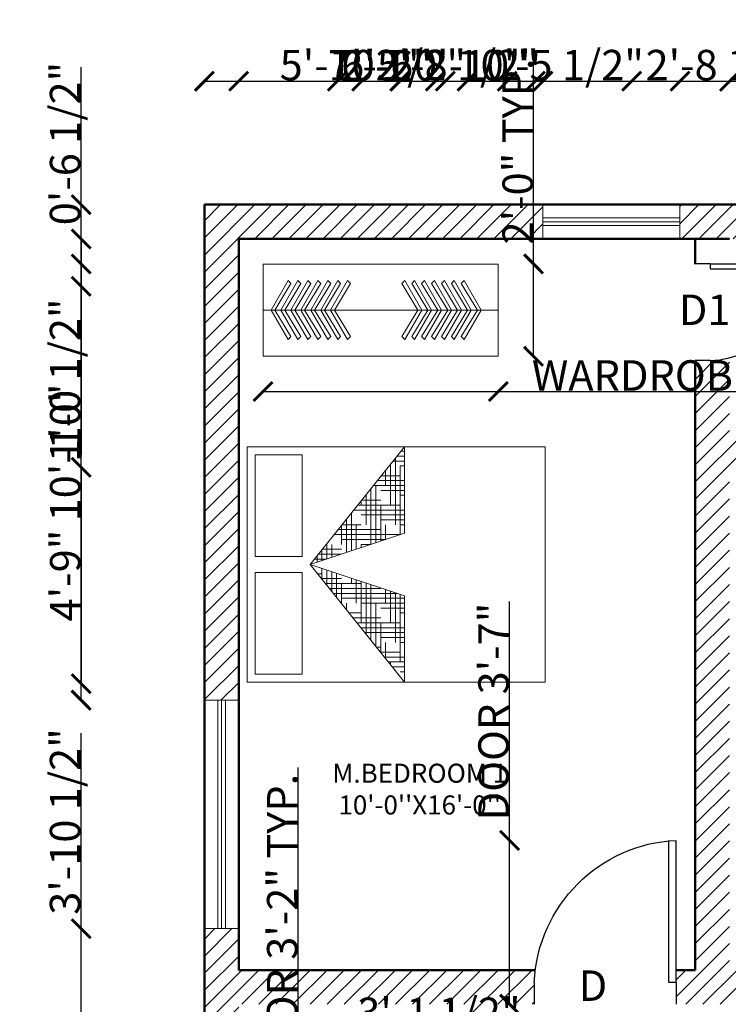
# Model space of a CAD drawing. Units: inches. Extents: x 1385 to 1778, y 1343 to 2100.
# Tile 4 of 6: x 1385 to 1571, y 1821 to 2079. Entities that reach past the tile are written whole.
import ezdxf

# ---------------------------------------------------------------- set-up
doc = ezdxf.new("R2010")
doc.units = ezdxf.units.IN
for name, color, linetype, lineweight in [('A-ANNO-DIMS', 2, 'Continuous', 18), ('A-ANNO-TEXT', 7, 'Continuous', 25), ('A-AREA-IDEN', 7, 'Continuous', 25), ('A-FURN', 8, 'Continuous', 18), ('A-WALL-PATT', 8, 'Continuous', 13), ('Door', 150, 'Continuous', 25), ('Wall', 7, 'Continuous', 50), ('Wardrobe', 114, 'Continuous', 18), ('Windows', 140, 'Continuous', 18)]:
    doc.layers.add(name, color=color, linetype=linetype, lineweight=lineweight)
doc.styles.get("Standard").update_dxf_attribs({"font": 'arial.ttf'})
doc.dimstyles.get("Standard").update_dxf_attribs({"dimtxt": 8, "dimasz": 5, "dimexe": 0.18, "dimexo": 0.0625, "dimgap": 0.09, "dimtad": 1, "dimdec": 1, "dimzin": 0, "dimdsep": 46, "dimlunit": 4, "dimtxsty": 'Standard', "dimblk": 'ARCHTICK', "dimcen": 0.09, "dimse1": 1, "dimse2": 1, "dimadec": 0, "dimazin": 0, "dimtfac": 1, "dimtdec": 1, "dimtofl": 0, "dimtmove": 0, "dimatfit": 3, "dimfxl": 1, "dimtolj": 1, "dimtzin": 0, "dimarcsym": 0})

# ---------------------------------------------------------------- blocks, each defined once
blk = doc.blocks.new('AP0B05')
for p, q in [((35, 100), (35, 880)), ((75, 100), (75, 878.9)), ((35, 100), (35, -20)), ((815, 100), (815, -20))]:
    blk.add_line(p, q)
blk.add_lwpolyline([(35, 100), (75, 100)])
blk.add_arc((-2.4, 62.6), 818.3, 2.6212, 87.3788)
blk = doc.blocks.new('*X10')
at = {"color": 0}
for p, q in [((20.25, 14.8125), (20.2772, 14.8125)), ((20.1739, 14.75), (20.2772, 14.75)), ((20.1875, 14.75), (20.1875, 14.7669)), ((20.199, 14.7812), (20.2772, 14.7812)), ((20.25, 14.3194), (20.25, 14.75)), ((20.1236, 14.6875), (20.25, 14.6875)), ((20.125, 14.5), (20.125, 14.6893)), ((20.1487, 14.7188), (20.2772, 14.7188)), ((20.1562, 14.625), (20.1562, 14.7281)), ((20.0938, 14.375), (20.0938, 14.6504)), ((20.0984, 14.6562), (20.125, 14.6562)), ((20.2188, 14.3091), (20.2188, 14.625)), ((20.25, 14.625), (20.2772, 14.625)), ((20.023, 14.5625), (20.2772, 14.5625)), ((20.0312, 14.2469), (20.0312, 14.5727)), ((20.0625, 14.2573), (20.0625, 14.6116)), ((20.125, 14.5938), (20.2772, 14.5938)), ((19.9727, 14.5), (20.25, 14.5)), ((19.9979, 14.5312), (20.2772, 14.5312)), ((20, 14.2366), (20, 14.5)), ((20.1875, 14.2987), (20.1875, 14.5)), ((19.9225, 14.4375), (20, 14.4375)), ((19.9476, 14.4688), (20.125, 14.4688)), ((20.25, 14.4375), (20.2772, 14.4375)), ((19.875, 14.25), (19.875, 14.3785)), ((19.9062, 14.375), (19.9062, 14.4174)), ((19.9688, 14.2262), (19.9688, 14.375)), ((20, 14.375), (20.2772, 14.375)), ((20.125, 14.4062), (20.2772, 14.4062)), ((20.1562, 14.2884), (20.1562, 14.375)), ((19.8219, 14.3125), (20.2291, 14.3125)), ((19.8438, 14.1848), (19.8438, 14.3397)), ((19.875, 14.3438), (20.2772, 14.3438)), ((19.7716, 14.25), (20, 14.25)), ((19.7812, 14.1641), (19.7812, 14.262)), ((19.7967, 14.2812), (20.125, 14.2812)), ((19.8125, 14.1744), (19.8125, 14.3008)), ((19.9375, 14.2159), (19.9375, 14.25)), ((19.7213, 14.1875), (19.75, 14.1875)), ((19.7465, 14.2188), (19.875, 14.2188)), ((19.75, 14.1537), (19.75, 14.2231)), ((19.7018, 14.0938), (19.7786, 14.0938)), ((19.7188, 14.0726), (19.7188, 14.1136)), ((19.7269, 14.0625), (19.8728, 14.0625)), ((19.75, 14.0338), (19.75, 14.1032)), ((19.7812, 13.9949), (19.7812, 14.0929)), ((19.8125, 14), (19.8125, 14.0825)), ((19.752, 14.0312), (19.875, 14.0312)), ((19.875, 13.8784), (19.875, 14)), ((19.9062, 13.8396), (19.9062, 14.0514)), ((19.9375, 13.8007), (19.9375, 14.0411)), ((19.9688, 13.875), (19.9688, 14.0307)), ((20, 14), (20, 14.0204)), ((20, 14), (20.0614, 14)), ((20.0625, 13.6454), (20.0625, 13.9996)), ((19.8275, 13.9375), (20.25, 13.9375)), ((19.875, 13.9688), (20.1557, 13.9688)), ((20.0938, 13.625), (20.0938, 13.9893)), ((20.125, 13.75), (20.125, 13.9789)), ((20.1562, 13.875), (20.1562, 13.9686)), ((20.25, 13.5), (20.25, 13.9375)), ((19.8526, 13.9062), (20.125, 13.9062)), ((19.8777, 13.875), (20, 13.875)), ((20.0312, 13.6842), (20.0312, 13.875)), ((20.2188, 13.4511), (20.2188, 13.875)), ((20.25, 13.875), (20.2772, 13.875)), ((20, 13.8125), (20.2772, 13.8125)), ((20.125, 13.8438), (20.2772, 13.8438)), ((19.9532, 13.7812), (20.2772, 13.7812)), ((19.9783, 13.75), (20.25, 13.75)), ((20, 13.723), (20, 13.75)), ((20.1875, 13.49), (20.1875, 13.75)), ((20.0035, 13.7188), (20.125, 13.7188)), ((20.25, 13.6875), (20.2772, 13.6875)), ((20.0789, 13.625), (20.2772, 13.625)), ((20.125, 13.6562), (20.2772, 13.6562)), ((20.1562, 13.5288), (20.1562, 13.625)), ((20.104, 13.5938), (20.2772, 13.5938)), ((20.1292, 13.5625), (20.25, 13.5625)), ((20.25, 13.5), (20.2772, 13.5)), ((20.2046, 13.4688), (20.2772, 13.4688)), ((20.2297, 13.4375), (20.2772, 13.4375)), ((20.2549, 13.4062), (20.2772, 13.4062))]:
    blk.add_line(p, q, dxfattribs=at)
blk = doc.blocks.new('MAT-P13')
for p, q in [((-0.75, 0), (0.75, 0)), ((-0.75, 0), (-0.75, -1.9)), ((0.75, 0), (0.75, -1.9)), ((-0.7, -0.05), (-0.7, -0.35)), ((-0.7, -0.05), (-0.05, -0.05)), ((-0.05, -0.35), (-0.05, -0.05)), ((0.05, -0.05), (0.7, -0.05)), ((0.05, -0.35), (0.05, -0.05)), ((0.7, -0.05), (0.7, -0.35)), ((-0.7, -0.35), (-0.05, -0.35)), ((0.05, -0.35), (0.7, -0.35)), ((-0.75, -1.0034), (0, -0.4)), ((0, -0.4), (-0.75, -1.0034)), ((0, -0.4), (-0.2, -1.0034)), ((0, -0.4), (0.2, -1.0034)), ((0, -0.4), (0.75, -1.0034)), ((-0.75, -1.0034), (-0.2, -1.0034)), ((0.2, -1.0034), (0.75, -1.0034)), ((0.75, -1.9), (-0.75, -1.9))]:
    blk.add_line(p, q)
at = {"xscale": -1, "rotation": 90}
blk.add_blockref('*X10', (14.1285, 19.2738), dxfattribs=at)
blk = doc.blocks.new('WARDROBE-DOUBLE')
blk.add_line((0, 12.12), (61.84, 12.12))
blk.add_lwpolyline([(0, 24.24), (61.84, 24.24), (61.84, 0), (0, 0)], close=True)
for points in [[(2.11, 12.12), (6.58, 19.87), (7.34, 19.08), (3.11, 12.12)], [(4.72, 12.12), (9.19, 19.87), (9.95, 19.08), (5.72, 12.12)], [(7.33, 12.12), (11.8, 19.87), (12.56, 19.08), (8.32, 12.12)], [(9.94, 12.12), (14.41, 19.87), (15.17, 19.08), (10.93, 12.12)], [(12.54, 12.12), (17.02, 19.87), (17.78, 19.08), (13.54, 12.12)], [(15.15, 12.12), (19.62, 19.87), (20.38, 19.08), (16.15, 12.12)], [(17.76, 12.12), (22.23, 19.87), (22.99, 19.08), (18.76, 12.12)], [(41.7, 12.12), (37.23, 19.87), (36.47, 19.08), (40.7, 12.12)], [(44.31, 12.12), (39.83, 19.87), (39.07, 19.08), (43.31, 12.12)], [(46.91, 12.12), (42.44, 19.87), (41.68, 19.08), (45.92, 12.12)], [(49.52, 12.12), (45.05, 19.87), (44.29, 19.08), (48.53, 12.12)], [(52.13, 12.12), (47.66, 19.87), (46.9, 19.08), (51.13, 12.12)], [(54.74, 12.12), (50.27, 19.87), (49.51, 19.08), (53.74, 12.12)], [(57.35, 12.12), (52.88, 19.87), (52.12, 19.08), (56.35, 12.12)], [(2.11, 12.12), (6.58, 4.38), (7.34, 5.17), (3.11, 12.12)], [(4.72, 12.12), (9.19, 4.38), (9.95, 5.17), (5.72, 12.12)], [(7.33, 12.12), (11.8, 4.38), (12.56, 5.17), (8.32, 12.12)], [(9.94, 12.12), (14.41, 4.38), (15.17, 5.17), (10.93, 12.12)], [(12.54, 12.12), (17.02, 4.38), (17.78, 5.17), (13.54, 12.12)], [(15.15, 12.12), (19.62, 4.38), (20.38, 5.17), (16.15, 12.12)], [(17.76, 12.12), (22.23, 4.38), (22.99, 5.17), (18.76, 12.12)], [(41.7, 12.12), (37.23, 4.38), (36.47, 5.17), (40.7, 12.12)], [(44.31, 12.12), (39.83, 4.38), (39.07, 5.17), (43.31, 12.12)], [(46.91, 12.12), (42.44, 4.38), (41.68, 5.17), (45.92, 12.12)], [(49.52, 12.12), (45.05, 4.38), (44.29, 5.17), (48.53, 12.12)], [(52.13, 12.12), (47.66, 4.38), (46.9, 5.17), (51.13, 12.12)], [(54.74, 12.12), (50.27, 4.38), (49.51, 5.17), (53.74, 12.12)], [(57.35, 12.12), (52.88, 4.38), (52.12, 5.17), (56.35, 12.12)]]:
    blk.add_lwpolyline(points)
blk = doc.blocks.new('WINDOW-GLAZING-36IN')
for p, q in [((0, 0), (0, 36)), ((1, 0), (1, 36)), ((2, 0), (2, 36))]:
    blk.add_line(p, q)
blk = doc.blocks.new('WINDOW-GLAZING-60IN')
for p, q in [((0, 0), (0, 60)), ((1, 0), (1, 60)), ((2, 0), (2, 60))]:
    blk.add_line(p, q)
blk = doc.blocks.new('_ArchTick')
at = {"color": 0, "linetype": 'ByBlock', "const_width": 0.15}
blk.add_lwpolyline([(-0.5, -0.5), (0.5, 0.5)], dxfattribs=at)
blk = doc.blocks.new('*D19')
at = {"layer": 'A-ANNO-DIMS', "color": 0, "lineweight": -2, "transparency": 16777216}
for p, q in [((1458.44, 1792.72), (1458.44, 1882.9)), ((1458.44, 1754.73), (1458.44, 1792.72))]:
    blk.add_line(p, q, dxfattribs=at)
at = {"layer": 'Defpoints', "color": 0, "transparency": 16777216}
for p in [(1458.44, 1792.72), (1464.14, 1792.72), (1464.14, 1754.73)]:
    blk.add_point(p, dxfattribs=at)
at = {"layer": 'A-ANNO-DIMS', "color": 0, "lineweight": -2, "transparency": 16777216, "xscale": 5, "yscale": 5, "zscale": 5}
for p, rotation in [((1458.44, 1792.72), 90), ((1458.44, 1754.73), 270)]:
    blk.add_blockref('_ArchTick', p, dxfattribs=dict(at, rotation=rotation))
at = {"layer": 'A-ANNO-DIMS', "color": 0, "transparency": 16777216, "insert": (1454.21, 1840.31), "char_height": 8, "attachment_point": 5, "rotation": 90}
blk.add_mtext('\\A1;DOOR 3\'-2" TYP.', dxfattribs=at)
blk = doc.blocks.new('*D21')
at = {"layer": 'A-ANNO-DIMS', "color": 0, "lineweight": -2, "transparency": 16777216}
for p, q in [((1513.99, 1863.79), (1513.99, 1926.47)), ((1513.99, 1820.73), (1513.99, 1863.79))]:
    blk.add_line(p, q, dxfattribs=at)
at = {"layer": 'Defpoints', "color": 0, "transparency": 16777216}
for p in [(1513.99, 1863.79), (1520.45, 1863.79), (1520.45, 1820.73)]:
    blk.add_point(p, dxfattribs=at)
at = {"layer": 'A-ANNO-DIMS', "color": 0, "lineweight": -2, "transparency": 16777216, "xscale": 5, "yscale": 5, "zscale": 5}
for p, rotation in [((1513.99, 1863.79), 90), ((1513.99, 1820.73), 270)]:
    blk.add_blockref('_ArchTick', p, dxfattribs=dict(at, rotation=rotation))
at = {"layer": 'A-ANNO-DIMS', "color": 0, "transparency": 16777216, "insert": (1509.76, 1897.63), "char_height": 8, "attachment_point": 5, "rotation": 90}
blk.add_mtext('\\A1;DOOR 3\'-7"', dxfattribs=at)
blk = doc.blocks.new('*D22')
at = {"layer": 'A-ANNO-DIMS', "color": 0, "lineweight": -2, "transparency": 16777216}
for p, q in [((1520.45, 1814.28), (1475.37, 1814.28)), ((1557.76, 1814.28), (1520.45, 1814.28))]:
    blk.add_line(p, q, dxfattribs=at)
at = {"layer": 'Defpoints', "color": 0, "transparency": 16777216}
for p in [(1520.45, 1820.73), (1557.76, 1820.73), (1520.45, 1814.28)]:
    blk.add_point(p, dxfattribs=at)
at = {"layer": 'A-ANNO-DIMS', "color": 0, "lineweight": -2, "transparency": 16777216, "xscale": 5, "yscale": 5, "zscale": 5, "rotation": 180}
blk.add_blockref('_ArchTick', (1520.45, 1814.28), dxfattribs=at)
at = {"layer": 'A-ANNO-DIMS', "color": 0, "lineweight": -2, "transparency": 16777216, "xscale": 5, "yscale": 5, "zscale": 5}
blk.add_blockref('_ArchTick', (1557.76, 1814.28), dxfattribs=at)
at = {"layer": 'A-ANNO-DIMS', "color": 0, "transparency": 16777216, "insert": (1495.41, 1818.51), "char_height": 8, "attachment_point": 5}
blk.add_mtext('\\A1;3\'-1 1/2"', dxfattribs=at)
blk = doc.blocks.new('*D37')
at = {"layer": 'A-ANNO-DIMS', "color": 0, "lineweight": -2, "transparency": 16777216}
for p, q in [((1449.17, 1981.63), (1511.01, 1981.63)), ((1511.01, 1981.63), (1634.21, 1981.63))]:
    blk.add_line(p, q, dxfattribs=at)
at = {"layer": 'Defpoints', "color": 0, "transparency": 16777216}
for p in [(1449.17, 1990.9), (1511.01, 1990.9), (1511.01, 1981.63)]:
    blk.add_point(p, dxfattribs=at)
at = {"layer": 'A-ANNO-DIMS', "color": 0, "lineweight": -2, "transparency": 16777216, "xscale": 5, "yscale": 5, "zscale": 5, "rotation": 180}
blk.add_blockref('_ArchTick', (1449.17, 1981.63), dxfattribs=at)
at = {"layer": 'A-ANNO-DIMS', "color": 0, "lineweight": -2, "transparency": 16777216, "xscale": 5, "yscale": 5, "zscale": 5}
blk.add_blockref('_ArchTick', (1511.01, 1981.63), dxfattribs=at)
at = {"layer": 'A-ANNO-DIMS', "color": 0, "transparency": 16777216, "insert": (1575.11, 1985.86), "char_height": 8, "attachment_point": 5}
blk.add_mtext('\\A1;WARDROBE 5\'-2" TYP.', dxfattribs=at)
blk = doc.blocks.new('*D38')
at = {"layer": 'A-ANNO-DIMS', "color": 0, "lineweight": -2, "transparency": 16777216}
for p, q in [((1520.29, 2015.15), (1520.29, 2069.23)), ((1520.29, 1990.9), (1520.29, 2015.15))]:
    blk.add_line(p, q, dxfattribs=at)
at = {"layer": 'Defpoints', "color": 0, "transparency": 16777216}
for p in [(1511.01, 2015.15), (1520.29, 2015.15), (1511.01, 1990.9)]:
    blk.add_point(p, dxfattribs=at)
at = {"layer": 'A-ANNO-DIMS', "color": 0, "lineweight": -2, "transparency": 16777216, "xscale": 5, "yscale": 5, "zscale": 5}
for p, rotation in [((1520.29, 2015.15), 90), ((1520.29, 1990.9), 270)]:
    blk.add_blockref('_ArchTick', p, dxfattribs=dict(at, rotation=rotation))
at = {"layer": 'A-ANNO-DIMS', "color": 0, "transparency": 16777216, "insert": (1516.11, 2044.69), "char_height": 8, "attachment_point": 5, "rotation": 90}
blk.add_mtext('\\A1;2\'-0" TYP.', dxfattribs=at)
blk = doc.blocks.new('*D51')
at = {"layer": 'A-ANNO-DIMS', "color": 0, "lineweight": -2, "transparency": 16777216}
blk.add_line((1433.77, 2063.14), (1522.75, 2063.14), dxfattribs=at)
at = {"layer": 'Defpoints', "color": 0, "transparency": 16777216}
for p in [(1522.75, 2063.14), (1433.77, 2030.73), (1522.75, 2030.73)]:
    blk.add_point(p, dxfattribs=at)
at = {"layer": 'A-ANNO-DIMS', "color": 0, "lineweight": -2, "transparency": 16777216, "xscale": 5, "yscale": 5, "zscale": 5, "rotation": 180}
blk.add_blockref('_ArchTick', (1433.77, 2063.14), dxfattribs=at)
at = {"layer": 'A-ANNO-DIMS', "color": 0, "lineweight": -2, "transparency": 16777216, "xscale": 5, "yscale": 5, "zscale": 5}
blk.add_blockref('_ArchTick', (1522.75, 2063.14), dxfattribs=at)
at = {"layer": 'A-ANNO-DIMS', "color": 0, "transparency": 16777216, "insert": (1478.26, 2067.3), "char_height": 8, "attachment_point": 5}
blk.add_mtext('\\A1;7\'-5"', dxfattribs=at)
blk = doc.blocks.new('*D52')
at = {"layer": 'A-ANNO-DIMS', "color": 0, "lineweight": -2, "transparency": 16777216}
for p, q in [((1558.75, 2063.14), (1591.32, 2063.14)), ((1591.32, 2063.14), (1636.55, 2063.14))]:
    blk.add_line(p, q, dxfattribs=at)
at = {"layer": 'Defpoints', "color": 0, "transparency": 16777216}
for p in [(1591.32, 2063.14), (1558.75, 2030.73), (1591.32, 2030.73)]:
    blk.add_point(p, dxfattribs=at)
at = {"layer": 'A-ANNO-DIMS', "color": 0, "lineweight": -2, "transparency": 16777216, "xscale": 5, "yscale": 5, "zscale": 5, "rotation": 180}
blk.add_blockref('_ArchTick', (1558.75, 2063.14), dxfattribs=at)
at = {"layer": 'A-ANNO-DIMS', "color": 0, "lineweight": -2, "transparency": 16777216, "xscale": 5, "yscale": 5, "zscale": 5}
blk.add_blockref('_ArchTick', (1591.32, 2063.14), dxfattribs=at)
at = {"layer": 'A-ANNO-DIMS', "color": 0, "transparency": 16777216, "insert": (1616.44, 2067.37), "char_height": 8, "attachment_point": 5}
blk.add_mtext('\\A1;2\'-8 1/2"', dxfattribs=at)
blk = doc.blocks.new('*D54')
at = {"layer": 'A-ANNO-DIMS', "color": 0, "lineweight": -2, "transparency": 16777216}
blk.add_line((1401.37, 1961.73), (1401.37, 1904.94), dxfattribs=at)
at = {"layer": 'Defpoints', "color": 0, "transparency": 16777216}
for p in [(1718.77, 1961.73), (1401.37, 1904.94), (1718.77, 1904.94)]:
    blk.add_point(p, dxfattribs=at)
at = {"layer": 'A-ANNO-DIMS', "color": 0, "lineweight": -2, "transparency": 16777216, "xscale": 5, "yscale": 5, "zscale": 5}
for p, rotation in [((1401.37, 1961.73), 90), ((1401.37, 1904.94), 270)]:
    blk.add_blockref('_ArchTick', p, dxfattribs=dict(at, rotation=rotation))
at = {"layer": 'A-ANNO-DIMS', "color": 0, "transparency": 16777216, "insert": (1397.19, 1933.34), "char_height": 8, "attachment_point": 5, "rotation": 90}
blk.add_mtext('\\A1;4\'-9"', dxfattribs=at)
blk = doc.blocks.new('*D56')
at = {"layer": 'A-ANNO-DIMS', "color": 0, "lineweight": -2, "transparency": 16777216}
blk.add_line((1401.37, 1900.6), (1401.37, 2030.73), dxfattribs=at)
at = {"layer": 'Defpoints', "color": 0, "transparency": 16777216}
for p in [(1401.37, 2030.73), (1433.77, 2030.73), (1433.77, 1900.6)]:
    blk.add_point(p, dxfattribs=at)
at = {"layer": 'A-ANNO-DIMS', "color": 0, "lineweight": -2, "transparency": 16777216, "xscale": 5, "yscale": 5, "zscale": 5}
for p, rotation in [((1401.37, 2030.73), 90), ((1401.37, 1900.6), 270)]:
    blk.add_blockref('_ArchTick', p, dxfattribs=dict(at, rotation=rotation))
at = {"layer": 'A-ANNO-DIMS', "color": 0, "transparency": 16777216, "insert": (1397.19, 1965.67), "char_height": 8, "attachment_point": 5, "rotation": 90}
blk.add_mtext('\\A1;10\'-10"', dxfattribs=at)
blk = doc.blocks.new('*D57')
at = {"layer": 'A-ANNO-DIMS', "color": 0, "lineweight": -2, "transparency": 16777216}
for p, q in [((1401.37, 1840.6), (1401.37, 1891.9)), ((1401.37, 1794.33), (1401.37, 1840.6))]:
    blk.add_line(p, q, dxfattribs=at)
at = {"layer": 'Defpoints', "color": 0, "transparency": 16777216}
for p in [(1401.37, 1840.6), (1433.77, 1840.6), (1433.77, 1794.33)]:
    blk.add_point(p, dxfattribs=at)
at = {"layer": 'A-ANNO-DIMS', "color": 0, "lineweight": -2, "transparency": 16777216, "xscale": 5, "yscale": 5, "zscale": 5}
for p, rotation in [((1401.37, 1840.6), 90), ((1401.37, 1794.33), 270)]:
    blk.add_blockref('_ArchTick', p, dxfattribs=dict(at, rotation=rotation))
at = {"layer": 'A-ANNO-DIMS', "color": 0, "transparency": 16777216, "insert": (1397.14, 1868.75), "char_height": 8, "attachment_point": 5, "rotation": 90}
blk.add_mtext('\\A1;3\'-10 1/2"', dxfattribs=at)
blk = doc.blocks.new('*D62')
at = {"layer": 'A-ANNO-DIMS', "color": 0, "lineweight": -2, "transparency": 16777216}
for p, q in [((1442.77, 2063.14), (1475.11, 2063.14)), ((1475.11, 2063.14), (1520.34, 2063.14))]:
    blk.add_line(p, q, dxfattribs=at)
at = {"layer": 'Defpoints', "color": 0, "transparency": 16777216}
for p in [(1475.11, 2063.14), (1442.77, 1391.73), (1475.11, 1391.73)]:
    blk.add_point(p, dxfattribs=at)
at = {"layer": 'A-ANNO-DIMS', "color": 0, "lineweight": -2, "transparency": 16777216, "xscale": 5, "yscale": 5, "zscale": 5, "rotation": 180}
blk.add_blockref('_ArchTick', (1442.77, 2063.14), dxfattribs=at)
at = {"layer": 'A-ANNO-DIMS', "color": 0, "lineweight": -2, "transparency": 16777216, "xscale": 5, "yscale": 5, "zscale": 5}
blk.add_blockref('_ArchTick', (1475.11, 2063.14), dxfattribs=at)
at = {"layer": 'A-ANNO-DIMS', "color": 0, "transparency": 16777216, "insert": (1500.22, 2067.37), "char_height": 8, "attachment_point": 5}
blk.add_mtext('\\A1;2\'-8 1/2"', dxfattribs=at)
blk = doc.blocks.new('*D63')
at = {"layer": 'A-ANNO-DIMS', "color": 0, "lineweight": -2, "transparency": 16777216}
for p, q in [((1475.11, 2063.14), (1485.11, 2063.14)), ((1485.11, 2063.14), (1517.77, 2063.14))]:
    blk.add_line(p, q, dxfattribs=at)
at = {"layer": 'Defpoints', "color": 0, "transparency": 16777216}
for p in [(1485.11, 2063.14), (1475.11, 1391.73), (1485.11, 1391.73)]:
    blk.add_point(p, dxfattribs=at)
at = {"layer": 'A-ANNO-DIMS', "color": 0, "lineweight": -2, "transparency": 16777216, "xscale": 5, "yscale": 5, "zscale": 5, "rotation": 180}
blk.add_blockref('_ArchTick', (1475.11, 2063.14), dxfattribs=at)
at = {"layer": 'A-ANNO-DIMS', "color": 0, "lineweight": -2, "transparency": 16777216, "xscale": 5, "yscale": 5, "zscale": 5}
blk.add_blockref('_ArchTick', (1485.11, 2063.14), dxfattribs=at)
at = {"layer": 'A-ANNO-DIMS', "color": 0, "transparency": 16777216, "insert": (1503.94, 2067.31), "char_height": 8, "attachment_point": 5}
blk.add_mtext('\\A1;0\'-10"', dxfattribs=at)
blk = doc.blocks.new('*D66')
at = {"layer": 'A-ANNO-DIMS', "color": 0, "lineweight": -2, "transparency": 16777216}
blk.add_line((1442.77, 2063.14), (1513.34, 2063.14), dxfattribs=at)
at = {"layer": 'Defpoints', "color": 0, "transparency": 16777216}
for p in [(1513.34, 2063.14), (1442.77, 1595.73), (1513.34, 1595.73)]:
    blk.add_point(p, dxfattribs=at)
at = {"layer": 'A-ANNO-DIMS', "color": 0, "lineweight": -2, "transparency": 16777216, "xscale": 5, "yscale": 5, "zscale": 5, "rotation": 180}
blk.add_blockref('_ArchTick', (1442.77, 2063.14), dxfattribs=at)
at = {"layer": 'A-ANNO-DIMS', "color": 0, "lineweight": -2, "transparency": 16777216, "xscale": 5, "yscale": 5, "zscale": 5}
blk.add_blockref('_ArchTick', (1513.34, 2063.14), dxfattribs=at)
at = {"layer": 'A-ANNO-DIMS', "color": 0, "transparency": 16777216, "insert": (1478.05, 2067.37), "char_height": 8, "attachment_point": 5}
blk.add_mtext('\\A1;5\'-10 1/2"', dxfattribs=at)
blk = doc.blocks.new('*D67')
at = {"layer": 'A-ANNO-DIMS', "color": 0, "lineweight": -2, "transparency": 16777216}
for p, q in [((1513.34, 2063.14), (1546.08, 2063.14)), ((1546.08, 2063.14), (1591.31, 2063.14))]:
    blk.add_line(p, q, dxfattribs=at)
at = {"layer": 'Defpoints', "color": 0, "transparency": 16777216}
for p in [(1546.08, 2063.14), (1513.34, 1595.73), (1546.08, 1595.73)]:
    blk.add_point(p, dxfattribs=at)
at = {"layer": 'A-ANNO-DIMS', "color": 0, "lineweight": -2, "transparency": 16777216, "xscale": 5, "yscale": 5, "zscale": 5, "rotation": 180}
blk.add_blockref('_ArchTick', (1513.34, 2063.14), dxfattribs=at)
at = {"layer": 'A-ANNO-DIMS', "color": 0, "lineweight": -2, "transparency": 16777216, "xscale": 5, "yscale": 5, "zscale": 5}
blk.add_blockref('_ArchTick', (1546.08, 2063.14), dxfattribs=at)
at = {"layer": 'A-ANNO-DIMS', "color": 0, "transparency": 16777216, "insert": (1571.19, 2067.37), "char_height": 8, "attachment_point": 5}
blk.add_mtext('\\A1;2\'-8 1/2"', dxfattribs=at)
blk = doc.blocks.new('*D69')
at = {"layer": 'A-ANNO-DIMS', "color": 0, "lineweight": -2, "transparency": 16777216}
blk.add_line((1442.77, 2063.14), (1520.74, 2063.14), dxfattribs=at)
at = {"layer": 'Defpoints', "color": 0, "transparency": 16777216}
for p in [(1520.74, 2063.14), (1442.77, 1829.73), (1520.74, 1829.73)]:
    blk.add_point(p, dxfattribs=at)
at = {"layer": 'A-ANNO-DIMS', "color": 0, "lineweight": -2, "transparency": 16777216, "xscale": 5, "yscale": 5, "zscale": 5, "rotation": 180}
blk.add_blockref('_ArchTick', (1442.77, 2063.14), dxfattribs=at)
at = {"layer": 'A-ANNO-DIMS', "color": 0, "lineweight": -2, "transparency": 16777216, "xscale": 5, "yscale": 5, "zscale": 5}
blk.add_blockref('_ArchTick', (1520.74, 2063.14), dxfattribs=at)
at = {"layer": 'A-ANNO-DIMS', "color": 0, "transparency": 16777216, "insert": (1481.75, 2067.31), "char_height": 8, "attachment_point": 5}
blk.add_mtext('\\A1;6\'-6"', dxfattribs=at)
blk = doc.blocks.new('*D70')
at = {"layer": 'A-ANNO-DIMS', "color": 0, "lineweight": -2, "transparency": 16777216}
for p, q in [((1571.77, 2063.14), (1578.09, 2063.14)), ((1578.09, 2063.14), (1623.18, 2063.14))]:
    blk.add_line(p, q, dxfattribs=at)
at = {"layer": 'Defpoints', "color": 0, "transparency": 16777216}
for p in [(1578.09, 2063.14), (1571.77, 1829.73), (1578.09, 1829.73)]:
    blk.add_point(p, dxfattribs=at)
at = {"layer": 'A-ANNO-DIMS', "color": 0, "lineweight": -2, "transparency": 16777216, "xscale": 5, "yscale": 5, "zscale": 5, "rotation": 180}
blk.add_blockref('_ArchTick', (1571.77, 2063.14), dxfattribs=at)
at = {"layer": 'A-ANNO-DIMS', "color": 0, "lineweight": -2, "transparency": 16777216, "xscale": 5, "yscale": 5, "zscale": 5}
blk.add_blockref('_ArchTick', (1578.09, 2063.14), dxfattribs=at)
at = {"layer": 'A-ANNO-DIMS', "color": 0, "transparency": 16777216, "insert": (1603.14, 2067.37), "char_height": 8, "attachment_point": 5}
blk.add_mtext('\\A1;0\'-6 1/2"', dxfattribs=at)
blk = doc.blocks.new('*D73')
at = {"layer": 'A-ANNO-DIMS', "color": 0, "lineweight": -2, "transparency": 16777216}
blk.add_line((1468.71, 2063.14), (1494.47, 2063.14), dxfattribs=at)
at = {"layer": 'Defpoints', "color": 0, "transparency": 16777216}
for p in [(1494.47, 2063.14), (1468.71, 1493.49), (1494.47, 1493.49)]:
    blk.add_point(p, dxfattribs=at)
at = {"layer": 'A-ANNO-DIMS', "color": 0, "lineweight": -2, "transparency": 16777216, "xscale": 5, "yscale": 5, "zscale": 5, "rotation": 180}
blk.add_blockref('_ArchTick', (1468.71, 2063.14), dxfattribs=at)
at = {"layer": 'A-ANNO-DIMS', "color": 0, "lineweight": -2, "transparency": 16777216, "xscale": 5, "yscale": 5, "zscale": 5}
blk.add_blockref('_ArchTick', (1494.47, 2063.14), dxfattribs=at)
at = {"layer": 'A-ANNO-DIMS', "color": 0, "transparency": 16777216, "insert": (1481.59, 2067.25), "char_height": 8, "attachment_point": 5}
blk.add_mtext('\\A1;2\'-2"', dxfattribs=at)
blk = doc.blocks.new('*D75')
at = {"layer": 'A-ANNO-DIMS', "color": 0, "lineweight": -2, "transparency": 16777216}
for p, q in [((1401.37, 2021.73), (1401.37, 2066.82)), ((1401.37, 2015.14), (1401.37, 2021.73))]:
    blk.add_line(p, q, dxfattribs=at)
at = {"layer": 'Defpoints', "color": 0, "transparency": 16777216}
for p in [(1401.37, 2021.73), (1571.77, 2021.73), (1571.77, 2015.14)]:
    blk.add_point(p, dxfattribs=at)
at = {"layer": 'A-ANNO-DIMS', "color": 0, "lineweight": -2, "transparency": 16777216, "xscale": 5, "yscale": 5, "zscale": 5}
for p, rotation in [((1401.37, 2021.73), 90), ((1401.37, 2015.14), 270)]:
    blk.add_blockref('_ArchTick', p, dxfattribs=dict(at, rotation=rotation))
at = {"layer": 'A-ANNO-DIMS', "color": 0, "transparency": 16777216, "insert": (1397.14, 2046.78), "char_height": 8, "attachment_point": 5, "rotation": 90}
blk.add_mtext('\\A1;0\'-6 1/2"', dxfattribs=at)
blk = doc.blocks.new('*D77')
at = {"layer": 'A-ANNO-DIMS', "color": 0, "lineweight": -2, "transparency": 16777216}
for p, q in [((1497.07, 2063.14), (1502.77, 2063.14)), ((1502.77, 2063.14), (1547.86, 2063.14))]:
    blk.add_line(p, q, dxfattribs=at)
at = {"layer": 'Defpoints', "color": 0, "transparency": 16777216}
for p in [(1502.77, 2063.14), (1497.07, 1760.73), (1502.77, 1760.73)]:
    blk.add_point(p, dxfattribs=at)
at = {"layer": 'A-ANNO-DIMS', "color": 0, "lineweight": -2, "transparency": 16777216, "xscale": 5, "yscale": 5, "zscale": 5, "rotation": 180}
blk.add_blockref('_ArchTick', (1497.07, 2063.14), dxfattribs=at)
at = {"layer": 'A-ANNO-DIMS', "color": 0, "lineweight": -2, "transparency": 16777216, "xscale": 5, "yscale": 5, "zscale": 5}
blk.add_blockref('_ArchTick', (1502.77, 2063.14), dxfattribs=at)
at = {"layer": 'A-ANNO-DIMS', "color": 0, "transparency": 16777216, "insert": (1527.82, 2067.37), "char_height": 8, "attachment_point": 5}
blk.add_mtext('\\A1;0\'-5 1/2"', dxfattribs=at)
blk = doc.blocks.new('*D79')
at = {"layer": 'A-ANNO-DIMS', "color": 0, "lineweight": -2, "transparency": 16777216}
blk.add_line((1760.18, 1784.73), (1760.18, 1820.73), dxfattribs=at)
at = {"layer": 'Defpoints', "color": 0, "transparency": 16777216}
for p in [(1508.77, 1820.73), (1760.18, 1820.73), (1508.77, 1784.73)]:
    blk.add_point(p, dxfattribs=at)
at = {"layer": 'A-ANNO-DIMS', "color": 0, "lineweight": -2, "transparency": 16777216, "xscale": 5, "yscale": 5, "zscale": 5}
for p, rotation in [((1760.18, 1820.73), 90), ((1760.18, 1784.73), 270)]:
    blk.add_blockref('_ArchTick', p, dxfattribs=dict(at, rotation=rotation))
at = {"layer": 'A-ANNO-DIMS', "color": 0, "transparency": 16777216, "insert": (1756, 1802.73), "char_height": 8, "attachment_point": 5, "rotation": 90}
blk.add_mtext('\\A1;3\'-0"', dxfattribs=at)
blk = doc.blocks.new('*D82')
at = {"layer": 'A-ANNO-DIMS', "color": 0, "lineweight": -2, "transparency": 16777216}
for p, q in [((1401.37, 2021.73), (1401.37, 2009.31)), ((1401.37, 2009.31), (1401.37, 1964.97))]:
    blk.add_line(p, q, dxfattribs=at)
at = {"layer": 'Defpoints', "color": 0, "transparency": 16777216}
for p in [(1646.77, 2021.73), (1401.37, 2009.31), (1646.77, 2009.31)]:
    blk.add_point(p, dxfattribs=at)
at = {"layer": 'A-ANNO-DIMS', "color": 0, "lineweight": -2, "transparency": 16777216, "xscale": 5, "yscale": 5, "zscale": 5}
for p, rotation in [((1401.37, 2021.73), 90), ((1401.37, 2009.31), 270)]:
    blk.add_blockref('_ArchTick', p, dxfattribs=dict(at, rotation=rotation))
at = {"layer": 'A-ANNO-DIMS', "color": 0, "transparency": 16777216, "insert": (1397.14, 1984.64), "char_height": 8, "attachment_point": 5, "rotation": 90}
blk.add_mtext('\\A1;1\'-0 1/2"', dxfattribs=at)

msp = doc.modelspace()

# ---------------------------------------------------------------- hatches: boundary and pattern name
at = {"layer": 'A-WALL-PATT', "transparency": 33554585}
h = msp.add_hatch(dxfattribs=at)
h.set_pattern_fill('ANSI31', color=256)
h.paths.add_polyline_path([(1522.75, 2030.73), (1433.77, 2030.73), (1433.77, 1900.6), (1442.77, 1900.6), (1442.77, 2021.73), (1522.75, 2021.73)])
h.paths.add_polyline_path([(1591.32, 2030.73), (1558.75, 2030.73), (1558.75, 2021.73), (1571.77, 2021.73), (1591.32, 2021.73)], flags=17)
h.paths.add_polyline_path([(1664.16, 2030.73), (1615.32, 2030.73), (1615.32, 2021.73), (1646.77, 2021.73), (1646.77, 1970.73), (1571.77, 1970.73), (1571.77, 1990.51, -0.048507), (1566.67, 1989.78), (1562.77, 1989.78), (1562.77, 1829.73), (1557.76, 1829.73), (1557.76, 1826.48), (1557.76, 1820.73), (1578.09, 1820.73), (1578.09, 1825.8), (1578.09, 1829.73), (1571.77, 1829.73), (1571.77, 1961.73), (1686.02, 1961.73), (1686.02, 1965.64, -0.048507), (1686.76, 1970.73), (1650.77, 1970.73), (1650.77, 2021.73), (1664.16, 2021.73)])
h.paths.add_polyline_path([(1727.77, 2030.73), (1688.16, 2030.73), (1688.16, 2021.73), (1718.77, 2021.73), (1718.77, 1970.73), (1711.39, 1970.73), (1711.39, 1965.64), (1711.39, 1961.73), (1718.77, 1961.73), (1718.77, 1904.94), (1727.77, 1904.94)])
h.paths.add_polyline_path([(1727.77, 1868.94), (1718.77, 1868.94), (1718.77, 1829.73), (1610.61, 1829.73, -0.028655), (1611.02, 1825.8), (1611.02, 1820.73), (1718.77, 1820.73), (1718.77, 1742.73), (1727.77, 1742.73)])
h.paths.add_polyline_path([(1520.45, 1826.48, -0.020905), (1520.74, 1829.73), (1442.77, 1829.73), (1442.77, 1840.6), (1433.77, 1840.6), (1433.77, 1794.33), (1442.77, 1794.33), (1442.77, 1820.73), (1502.77, 1820.73), (1502.77, 1760.73), (1497.07, 1760.73), (1497.07, 1759.8), (1497.07, 1754.73), (1508.77, 1754.73), (1508.77, 1778.73), (1562.77, 1778.73), (1562.77, 1656.82), (1571.77, 1656.82), (1571.77, 1784.73), (1508.77, 1784.73), (1508.77, 1820.73), (1520.45, 1820.73)])
h.paths.add_polyline_path([(1442.77, 1770.33), (1433.77, 1770.33), (1433.77, 1683.46), (1442.77, 1683.46)], flags=17)
h.paths.add_polyline_path([(1656.16, 1603.19, -0.007591), (1656.26, 1604.73), (1622.77, 1604.73), (1622.77, 1595.73), (1656.16, 1595.73)])
h.paths.add_polyline_path([(1727.77, 1682.73), (1718.77, 1682.73), (1718.77, 1604.73), (1704.65, 1604.73), (1704.65, 1603.19), (1704.65, 1595.73), (1727.77, 1595.73)])
h.paths.add_polyline_path([(1513.34, 1595.73), (1513.34, 1604.73), (1442.77, 1604.73), (1442.77, 1647.46), (1433.77, 1647.46), (1433.77, 1531.33), (1442.77, 1531.33), (1442.77, 1595.73)])
h.paths.add_polyline_path([(1546.08, 1604.73), (1546.08, 1595.73), (1577.77, 1595.73), (1577.77, 1472.73), (1541.77, 1472.73), (1541.77, 1523.73), (1537.77, 1523.73), (1537.77, 1472.73), (1442.77, 1472.73), (1442.77, 1495.33), (1433.77, 1495.33), (1433.77, 1382.73), (1586.77, 1382.73), (1586.77, 1391.73), (1442.77, 1391.73), (1442.77, 1463.73), (1586.77, 1463.73), (1586.77, 1604.73)])

# ---------------------------------------------------------------- linework, layer by layer
at = {"layer": 'Wall'}
for p, q in [((1433.77, 2030.73), (1727.77, 2030.73)), ((1433.77, 2030.73), (1433.77, 1382.73)), ((1442.77, 2021.73), (1571.77, 2021.73)), ((1442.77, 2021.73), (1442.77, 1829.73)), ((1562.77, 2021.73), (1562.77, 2015.14)), ((1562.77, 1989.78), (1562.77, 1829.73)), ((1442.77, 1829.73), (1520.74, 1829.73)), ((1557.76, 1829.73), (1562.77, 1829.73))]:
    msp.add_line(p, q, dxfattribs=at)
at = {"layer": 'Windows'}
for points in [[(1522.75, 2030.73), (1558.75, 2030.73), (1558.75, 2021.73), (1522.75, 2021.73)], [(1433.77, 1840.6), (1433.77, 1900.6), (1442.77, 1900.6), (1442.77, 1840.6)]]:
    msp.add_lwpolyline(points, close=True, dxfattribs=at)

# ---------------------------------------------------------------- block references
at = {"layer": 'A-FURN', "xscale": 41.19665858361839, "yscale": 41.19665858361839, "zscale": 41.19665858361839, "rotation": 90}
msp.add_blockref('MAT-P13', (1445.04, 1936.23), dxfattribs=at)
at = {"layer": 'Door', "xscale": 0.0325161801220908, "yscale": 0.0325161801220908, "zscale": 0.0325161801220908, "rotation": 270}
msp.add_blockref('AP0B05', (1563.42, 2016.28), dxfattribs=at)
at = {"layer": 'Door', "xscale": -0.0478384768610727, "yscale": 0.0478384768610727, "zscale": 0.0478384768610727}
msp.add_blockref('AP0B05', (1559.44, 1821.69), dxfattribs=at)
at = {"layer": 'Wardrobe'}
msp.add_blockref('WARDROBE-DOUBLE', (1449.17, 1990.9), dxfattribs=at)
at = {"layer": 'Windows'}
for name, p, rotation in [('WINDOW-GLAZING-36IN', (1558.75, 2025.23), 90.0000000000023), ('WINDOW-GLAZING-60IN', (1439.27, 1900.6), 180)]:
    msp.add_blockref(name, p, dxfattribs=dict(at, rotation=rotation))

# ---------------------------------------------------------------- texts
at = {"layer": 'A-ANNO-TEXT'}
for s, p in [('D1', (1558.46, 1999.11)), ('D', (1532.13, 1821.63))]:
    msp.add_text(s, height=8, dxfattribs=at).set_placement(p)
at = {"layer": 'A-AREA-IDEN', "insert": (1465.21, 1883.92), "char_height": 5, "attachment_point": 1}
msp.add_mtext_dynamic_manual_height_columns("\\pxqc;M.BEDROOM 1\\P10'-0''X16'-0''", width=50.3036, gutter_width=12.5, heights=[0], dxfattribs=at)

# ---------------------------------------------------------------- dimensions: what is measured, and where the dimension line sits
at = {"layer": 'A-ANNO-DIMS'}
for base, p1, p2, picture, middle in [((1475.11, 2063.14), (1442.77, 1391.73), (1475.11, 1391.73), '*D62', (1500.22, 2067.37)), ((1513.34, 2063.14), (1442.77, 1595.73), (1513.34, 1595.73), '*D66', (1478.05, 2067.37)), ((1502.77, 2063.14), (1497.07, 1760.73), (1502.77, 1760.73), '*D77', (1527.82, 2067.37)), ((1546.08, 2063.14), (1513.34, 1595.73), (1546.08, 1595.73), '*D67', (1571.19, 2067.37)), ((1591.32, 2063.14), (1558.75, 2030.73), (1591.32, 2030.73), '*D52', (1616.44, 2067.37)), ((1578.09, 2063.14), (1571.77, 1829.73), (1578.09, 1829.73), '*D70', (1603.14, 2067.37)), ((1522.75, 2063.14), (1433.77, 2030.73), (1522.75, 2030.73), '*D51', (1478.26, 2067.3)), ((1520.74, 2063.14), (1442.77, 1829.73), (1520.74, 1829.73), '*D69', (1481.75, 2067.31)), ((1494.47, 2063.14), (1468.71, 1493.49), (1494.47, 1493.49), '*D73', (1481.59, 2067.25)), ((1485.11, 2063.14), (1475.11, 1391.73), (1485.11, 1391.73), '*D63', (1503.94, 2067.31))]:
    dim = msp.add_linear_dim(base=base, p1=p1, p2=p2, dimstyle='Standard', override={"dimdec": 1, "dimlfac": 1, "dimrnd": 0, "dimzin": 1, "dimdsep": 46, "dimlunit": 4, "dimfrac": 2}, dxfattribs=at)
    dim.commit()
    dim.dimension.update_dxf_attribs({"geometry": picture, "text_midpoint": middle})
for base, p1, p2, text, picture, middle in [((1520.2888, 2015.1462), (1511.0124, 1990.9033), (1511.0124, 2015.1462), '<> TYP.', '*D38', (1516.1142, 2044.6864)), ((1513.99, 1863.79), (1520.45, 1820.73), (1520.45, 1863.79), 'DOOR <>', '*D21', (1509.76, 1897.63)), ((1458.44, 1792.72), (1464.14, 1754.73), (1464.14, 1792.72), 'DOOR <> TYP.', '*D19', (1454.21, 1840.31))]:
    dim = msp.add_linear_dim(base=base, p1=p1, p2=p2, angle=90, text=text, dimstyle='Standard', override={"dimdec": 1, "dimlfac": 1, "dimrnd": 0, "dimzin": 1, "dimdsep": 46, "dimlunit": 4, "dimfrac": 2}, dxfattribs=at)
    dim.commit()
    dim.dimension.update_dxf_attribs({"geometry": picture, "text_midpoint": middle})
for base, p1, p2, angle, picture, middle in [((1401.37, 2021.73), (1571.77, 2015.14), (1571.77, 2021.73), 90, '*D75', (1397.14, 2046.78)), ((1401.37, 2030.73), (1433.77, 1900.6), (1433.77, 2030.73), 90, '*D56', (1397.19, 1965.67)), ((1401.37, 2009.31), (1646.77, 2021.73), (1646.77, 2009.31), 90, '*D82', (1397.14, 1984.64)), ((1401.37, 1904.94), (1718.77, 1961.73), (1718.77, 1904.94), 90, '*D54', (1397.19, 1933.34)), ((1401.37, 1840.6), (1433.77, 1794.33), (1433.77, 1840.6), 90, '*D57', (1397.14, 1868.75)), ((1520.45, 1814.28), (1557.76, 1820.73), (1520.45, 1820.73), 180, '*D22', (1495.41, 1818.51)), ((1760.18, 1820.73), (1508.77, 1784.73), (1508.77, 1820.73), 90, '*D79', (1756, 1802.73))]:
    dim = msp.add_linear_dim(base=base, p1=p1, p2=p2, angle=angle, dimstyle='Standard', override={"dimdec": 1, "dimlfac": 1, "dimrnd": 0, "dimzin": 1, "dimdsep": 46, "dimlunit": 4, "dimfrac": 2}, dxfattribs=at)
    dim.commit()
    dim.dimension.update_dxf_attribs({"geometry": picture, "text_midpoint": middle})
dim = msp.add_linear_dim(base=(1511.01, 1981.63), p1=(1449.17, 1990.9), p2=(1511.01, 1990.9), text='WARDROBE <> TYP.', dimstyle='Standard', override={"dimdec": 1, "dimlfac": 1, "dimrnd": 0, "dimzin": 1, "dimdsep": 46, "dimlunit": 4, "dimfrac": 2}, dxfattribs=at)
dim.commit()
dim.dimension.update_dxf_attribs({"geometry": '*D37', "text_midpoint": (1575.11, 1985.86)})

doc.saveas('drawing.dxf')
